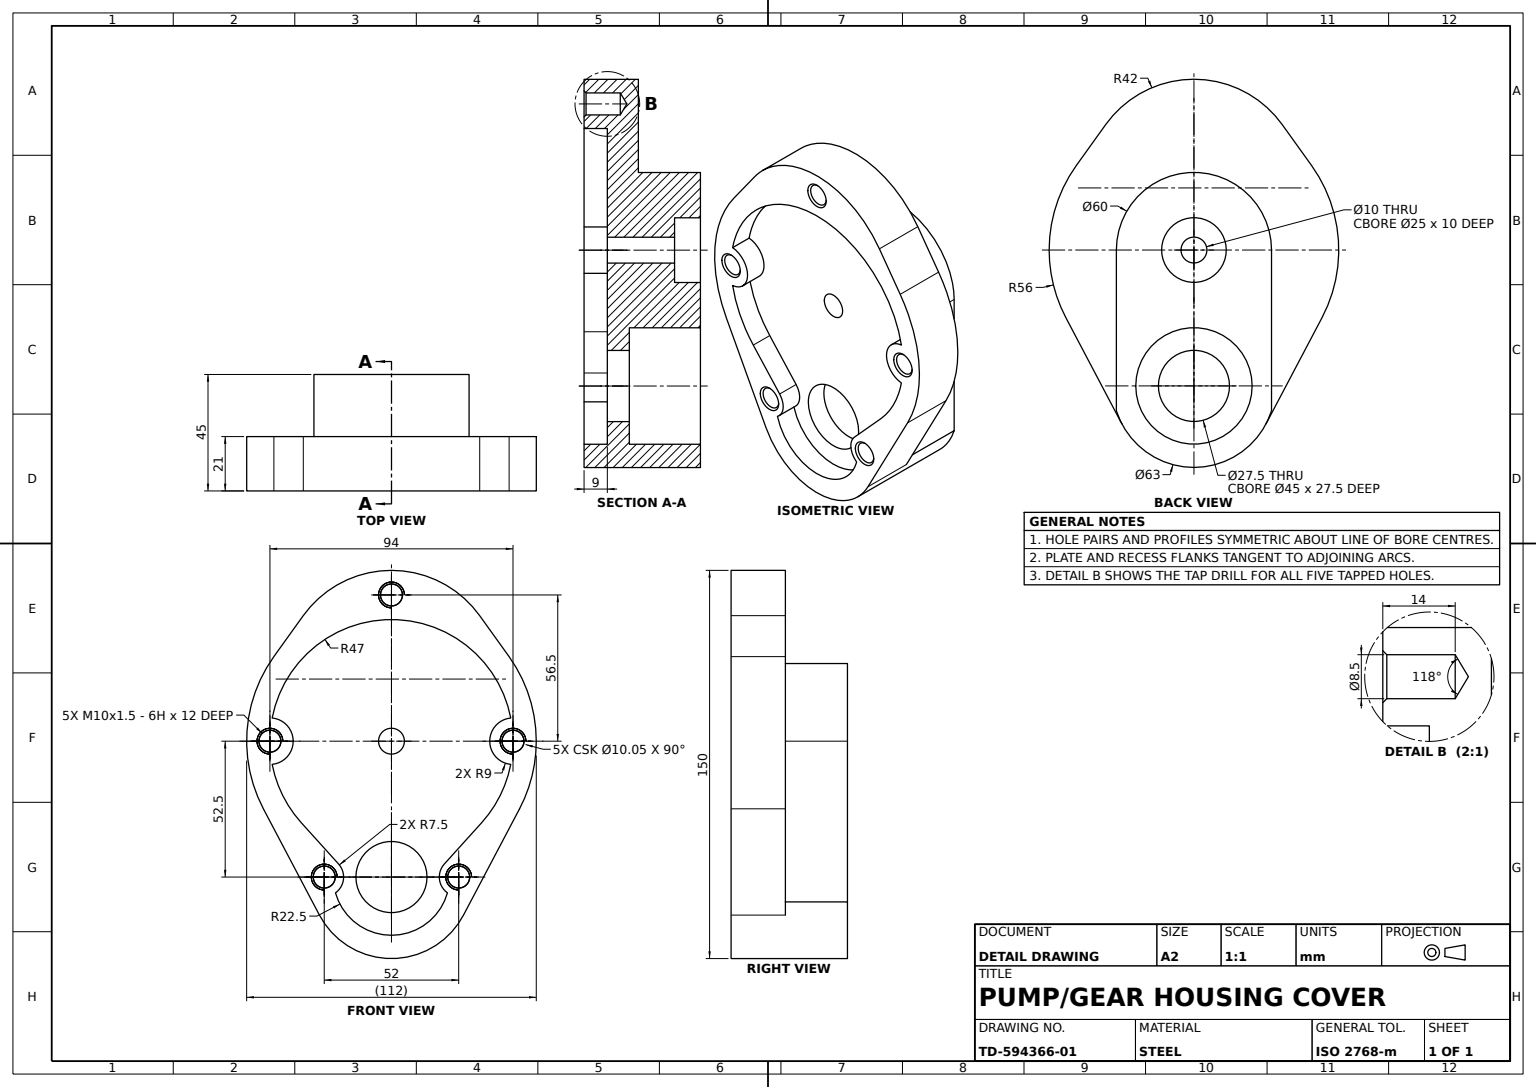
SolidWorks part; units mm, degrees
material "Plain Carbon Steel"
ref_plane "Front Plane" through (0, 0, 0) normal (0, 0, 1) x (1, 0, 0)
ref_plane "Top Plane" through (0, 0, 0) normal (0, 1, 0) x (1, 0, 0)
ref_plane "Right Plane" through (0, 0, 0) normal (1, 0, 0) x (0, 0, -1)
sketch "Plate Profile Sketch" plane through (0, 0, 0) normal (1, 0, 0) x (0, 0, -1)
  line L1 (-56, 66) -> (56, 66)
  line L2 (-56, 66) -> (-56, -84)
  line L3 (-56, -84) -> (56, -84)
  line L4 (56, 66) -> (56, -84)
  point P0 (0, 0)
  dimension "D1" = 150
  dimension "D2" = 112
  dimension "D3" = 84
  dimension "D4" = 56
extrude "Cover Plate 21mm" add sketch "Plate Profile Sketch" along normal blind 21
sketch "Inner Recess Sketch" plane through (21, 0, 0) normal (1, 0, 0) x (0, 0, -1)
  line L0 (0, 66) -> (0, -84) construction
  line L1 (56, 66) -> (-56, 66) construction
  line L2 (-56, -84) -> (56, -84) construction
  line L3 (-49.5283, -26.1333) -> (-27.8596, -67.2)
  line L4 (-45.485, 32.6667) -> (-34.1138, 48.5)
  line L5 (49.5283, -26.1333) -> (27.8596, -67.2)
  line L6 (45.485, 32.6667) -> (34.1138, 48.5)
  arc A0 (34.1138, 48.5) -> (-34.1138, 48.5) centre (0, 24) ccw
  arc A1 (-27.8596, -67.2) -> (27.8596, -67.2) centre (0, -52.5) ccw
  arc A2 (-45.485, 32.6667) -> (-49.5283, -26.1333) centre (0, 0) ccw
  arc A3 (49.5283, -26.1333) -> (45.485, 32.6667) centre (0, 0) ccw
  dimension "D1" = 84
  dimension "D2" = 63
  dimension "D3" = 112
extrude "Inner Recess Cut" cut sketch "Inner Recess Sketch" against normal blind 21 flip side to cut
sketch "Bore Boss Sketch" plane through (0, 0, 0) normal (-1, 0, 0) x (0, 0, 1)
  line L0 (0, 0) -> (0, -84) construction
  line L1 (30, 0) -> (30, -62.1047)
  line L2 (-30, 0) -> (-30, -62.1047)
  line L3 (-30, 0) -> (30, 0) construction
  arc A0 (-27.8596, -67.2) -> (27.8596, -67.2) centre (0, -52.5) ccw construction
  arc A1 (30, 0) -> (-30, 0) centre (0, 0) ccw
  arc A3 (-30, -62.1047) -> (30, -62.1047) centre (0, -52.5) ccw
  point P6 (0, 0)
  dimension "D1" = 60
extrude "Bore Boss Ø60" add sketch "Bore Boss Sketch" along normal blind 24
sketch "Face Recess Sketch" plane through (21, 0, 0) normal (1, 0, 0) x (0, 0, -1)
  line L0 (0, 0) -> (0, -52.5) construction
  line L1 (-26, -52.5) -> (0, -52.5) construction
  line L2 (-20.4378, -47.4689) -> (-34.8564, -31.5283)
  line L3 (20.4378, -47.4689) -> (34.8564, -31.5283)
  arc A0 (34.8564, -31.5283) -> (46.1383, -8.9587) centre (0, 0) ccw
  arc A2 (20.4378, -47.4689) -> (21.6538, -58.6124) centre (26, -52.5) ccw
  arc A3 (-20.4378, -47.4689) -> (-21.6538, -58.6124) centre (-26, -52.5) cw
  arc A4 (-46.1383, -8.9587) -> (-46.1383, 8.9587) centre (-47, 0) ccw
  arc A5 (46.1383, -8.9587) -> (46.1383, 8.9587) centre (47, 0) cw
  arc A6 (46.1383, 8.9587) -> (-46.1383, 8.9587) centre (0, 0) ccw
  arc A7 (-21.6538, -58.6124) -> (21.6538, -58.6124) centre (0, -52.5) ccw
  arc A8 (-46.1383, -8.9587) -> (-34.8564, -31.5283) centre (0, 0) ccw
  dimension "D1" = 94
  dimension "D3" = 7.5
  dimension "D5" = 9
  dimension "D6" = 22.5
  dimension "D2" = 52.5
  dimension "D4" = 52
extrude "Face Recess 9mm" cut sketch "Face Recess Sketch" against normal blind 9
hole_wizard "M10 Tapped Holes" positions "Sketch5" profile "Sketch6" tap size "M10" standard "ISO"
sketch "Sketch5" plane through (21, 0, 0) normal (1, 0, 0) x (0, 0, -1)
  line L0 (0, 56.5) -> (0, 0) construction
  point P0 (-47, 0)
  point P3 (47, 0)
  point P6 (26, -52.5)
  point P9 (-26, -52.5)
  point P12 (0, 56.5)
  dimension "D1" = 56.5
sketch "Sketch6" plane through (21, 0, 47) normal (0, 1, 0) x (0, 0, -1)
  line L0 (0, 0) -> (0, 16.5537)
  line L1 (0, 16.5537) -> (4.25, 14)
  line L2 (4.25, 14) -> (4.25, 0.775)
  line L3 (4.25, 0.775) -> (5.025, 0)
  line L5 (5.025, 0) -> (0, 0)
  line L6 (-4.25, 0.775) -> (-5.025, 0) construction
  line L10 (0, 16.5537) -> (-4.25, 14) construction
  line L11 (0, -6.35) -> (0, 107.95) construction
  dimension "Tap Drill Dia." = 8.5
  dimension "Tap Drill Depth" = 14
  dimension "Near C'Sink Dia." = 10.05
  dimension "Near C'Sink Angle" = 90
  dimension "Drill Angle" = 118
cosmetic thread "Hole Thread1" parameters "D1"=12, "D2"=10
cosmetic thread "Hole Thread2" parameters "D1"=12, "D2"=10
cosmetic thread "Hole Thread3" parameters "D1"=12, "D2"=10
cosmetic thread "Hole Thread4" parameters "D1"=12, "D2"=10
cosmetic thread "Hole Thread5" parameters "D1"=12, "D2"=10
hole_wizard "Counterbored Hole Ø10" positions "Sketch7" profile "Sketch8" legacy
sketch "Sketch7" plane through (-24, 0, 0) normal (-1, 0, 0) x (0, 0, 1)
  point P0 (0, 0)
sketch "Sketch8" plane through (-24, 0, 0) normal (0, 1, 0) x (0, 0, 1)
  line L0 (0, 0) -> (0, 100)
  line L1 (0, 100) -> (5, 100)
  line L2 (5, 100) -> (5, 10)
  line L3 (5, 10) -> (12.5, 10)
  line L4 (12.5, 10) -> (12.5, 0)
  line L5 (12.5, 0) -> (0, 0)
  line L6 (0, 110) -> (0, -10) construction
  dimension "Diameter" = 10
  dimension "Depth" = 100
  dimension "C-Bore Diameter" = 25
  dimension "C-Bore Depth" = 10
hole_wizard "Counterbored Bore Ø27.5" positions "Sketch9" profile "Sketch10" legacy
sketch "Sketch9" plane through (-24, 0, 0) normal (-1, 0, 0) x (0, 0, 1)
  point P0 (0, -52.5)
sketch "Sketch10" plane through (-24, -52.5, 0) normal (0, 1, 0) x (0, 0, 1)
  line L0 (0, 0) -> (0, 100)
  line L1 (0, 100) -> (13.75, 100)
  line L2 (13.75, 100) -> (13.75, 27.5)
  line L3 (13.75, 27.5) -> (22.5, 27.5)
  line L4 (22.5, 27.5) -> (22.5, 0)
  line L5 (22.5, 0) -> (0, 0)
  line L6 (0, 110) -> (0, -10) construction
  dimension "Diameter" = 27.5
  dimension "Depth" = 100
  dimension "C-Bore Diameter" = 45
  dimension "C-Bore Depth" = 27.5
